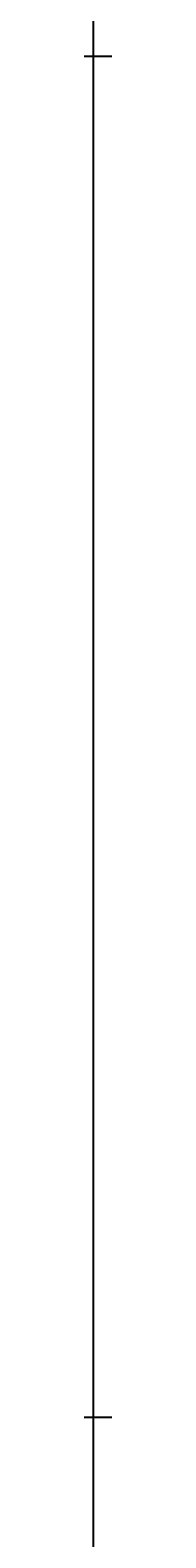
# Model space of a CAD drawing. Units: inches. Extents: x 35362 to 73946, y 43607 to 67532.
# Tile 43 of 134: x 48374 to 48377, y 46091 to 46564. Entities that reach past the tile are written whole.
import ezdxf

# ---------------------------------------------------------------- set-up
doc = ezdxf.new("R2010")
doc.units = ezdxf.units.IN
doc.header["$MEASUREMENT"] = 0
doc.layers.add('A-ANNO-DIMS', color=2, linetype='Continuous', lineweight=18)
doc.styles.get("Standard").update_dxf_attribs({"font": 'arial.ttf'})
doc.dimstyles.get("Standard").update_dxf_attribs({"dimtxt": 0.18, "dimasz": 0.18, "dimexe": 0.18, "dimexo": 0.0625, "dimgap": 0.09, "dimtad": 0, "dimtih": 1, "dimtoh": 1, "dimdec": 4, "dimzin": 0, "dimdsep": 46, "dimtxsty": 'Standard', "dimcen": 0.09, "dimadec": 0, "dimazin": 0, "dimtfac": 1, "dimtdec": 4, "dimtofl": 0, "dimtmove": 0, "dimatfit": 3, "dimfxl": 1, "dimtolj": 1, "dimtzin": 0, "dimarcsym": 0})

# ---------------------------------------------------------------- blocks, each defined once
blk = doc.blocks.new('*D5')
at = {"layer": 'A-ANNO-DIMS', "color": 0, "lineweight": -2, "transparency": 16777216}
for p, q in [((37121.95, 46919.32), (37121.95, 43606.68)), ((69871.5, 45449.83), (69871.5, 43606.68)), ((37122.13, 43606.86), (53496.29, 43606.86)), ((69871.32, 43606.86), (53497.15, 43606.86))]:
    blk.add_line(p, q, dxfattribs=at)
at = {"layer": 'A-ANNO-DIMS', "color": 0, "transparency": 16777216}
for points in [[(37122.13, 43606.89), (37122.13, 43606.83), (37121.95, 43606.86)], [(69871.32, 43606.89), (69871.32, 43606.83), (69871.5, 43606.86)]]:
    blk.add_solid(points, dxfattribs=at)
at = {"layer": 'Defpoints', "color": 0, "transparency": 16777216}
for p in [(37121.95, 46919.38), (69871.5, 45449.89), (69871.5, 43606.86)]:
    blk.add_point(p, dxfattribs=at)
at = {"layer": 'A-ANNO-DIMS', "color": 0, "transparency": 16777216, "insert": (53496.72, 43606.86), "char_height": 0.18, "attachment_point": 5}
blk.add_mtext('\\A1;32750', dxfattribs=at)
blk = doc.blocks.new('*D11')
at = {"layer": 'A-ANNO-DIMS', "color": 0, "lineweight": -2, "transparency": 16777216}
for p, q in [((47978.66, 56028.77), (47978.66, 43606.68)), ((53109.76, 56028.77), (53109.76, 43606.68)), ((47978.84, 43606.86), (50543.87, 43606.86)), ((53109.58, 43606.86), (50544.55, 43606.86))]:
    blk.add_line(p, q, dxfattribs=at)
at = {"layer": 'A-ANNO-DIMS', "color": 0, "transparency": 16777216}
for points in [[(47978.84, 43606.89), (47978.84, 43606.83), (47978.66, 43606.86)], [(53109.58, 43606.89), (53109.58, 43606.83), (53109.76, 43606.86)]]:
    blk.add_solid(points, dxfattribs=at)
at = {"layer": 'Defpoints', "color": 0, "transparency": 16777216}
for p in [(47978.66, 56028.84), (53109.76, 56028.84), (53109.76, 43606.86)]:
    blk.add_point(p, dxfattribs=at)
at = {"layer": 'A-ANNO-DIMS', "color": 0, "transparency": 16777216, "insert": (50544.21, 43606.86), "char_height": 0.18, "attachment_point": 5}
blk.add_mtext('\\A1;5131', dxfattribs=at)
blk = doc.blocks.new('*D13')
at = {"layer": 'A-ANNO-DIMS', "color": 0, "lineweight": -2, "transparency": 16777216}
for p, q in [((48373.49, 51694.02), (48373.49, 43606.68)), ((51029.04, 51694.02), (51029.04, 43606.68)), ((48373.67, 43606.86), (49700.8, 43606.86)), ((51028.86, 43606.86), (49701.73, 43606.86))]:
    blk.add_line(p, q, dxfattribs=at)
at = {"layer": 'A-ANNO-DIMS', "color": 0, "transparency": 16777216}
for points in [[(48373.67, 43606.89), (48373.67, 43606.83), (48373.49, 43606.86)], [(51028.86, 43606.89), (51028.86, 43606.83), (51029.04, 43606.86)]]:
    blk.add_solid(points, dxfattribs=at)
at = {"layer": 'Defpoints', "color": 0, "transparency": 16777216}
for p in [(48373.49, 51694.09), (51029.04, 51694.09), (51029.04, 43606.86)]:
    blk.add_point(p, dxfattribs=at)
at = {"layer": 'A-ANNO-DIMS', "color": 0, "transparency": 16777216, "insert": (49701.27, 43606.86), "char_height": 0.18, "attachment_point": 5}
blk.add_mtext('\\A1;2655.6', dxfattribs=at)
blk = doc.blocks.new('*D67')
at = {"layer": 'A-ANNO-DIMS', "color": 0, "lineweight": -2, "transparency": 16777216}
for p, q in [((56873.54, 53351.53), (35361.77, 53351.53)), ((35361.95, 53351.35), (35361.95, 49400.89)), ((35361.95, 45450.07), (35361.95, 49400.53)), ((53793.58, 45449.89), (35361.77, 45449.89))]:
    blk.add_line(p, q, dxfattribs=at)
at = {"layer": 'A-ANNO-DIMS', "color": 0, "transparency": 16777216}
for points in [[(35361.92, 53351.35), (35361.98, 53351.35), (35361.95, 53351.53)], [(35361.92, 45450.07), (35361.98, 45450.07), (35361.95, 45449.89)]]:
    blk.add_solid(points, dxfattribs=at)
at = {"layer": 'Defpoints', "color": 0, "transparency": 16777216}
for p in [(35361.95, 53351.53), (56873.6, 53351.53), (53793.64, 45449.89)]:
    blk.add_point(p, dxfattribs=at)
at = {"layer": 'A-ANNO-DIMS', "color": 0, "transparency": 16777216, "insert": (35361.95, 49400.71), "char_height": 0.18, "attachment_point": 5}
blk.add_mtext('\\A1;7901.6', dxfattribs=at)
blk = doc.blocks.new('*D76')
at = {"layer": 'A-ANNO-DIMS', "color": 0, "lineweight": -2, "transparency": 16777216}
for p, q in [((54052.84, 46555.29), (35361.77, 46555.29)), ((35361.95, 46555.11), (35361.95, 46342.27)), ((35361.95, 46129.06), (35361.95, 46341.9)), ((53793.58, 46128.88), (35361.77, 46128.88))]:
    blk.add_line(p, q, dxfattribs=at)
at = {"layer": 'A-ANNO-DIMS', "color": 0, "transparency": 16777216}
for points in [[(35361.92, 46555.11), (35361.98, 46555.11), (35361.95, 46555.29)], [(35361.92, 46129.06), (35361.98, 46129.06), (35361.95, 46128.88)]]:
    blk.add_solid(points, dxfattribs=at)
at = {"layer": 'Defpoints', "color": 0, "transparency": 16777216}
for p in [(35361.95, 46555.29), (54052.9, 46555.29), (53793.64, 46128.88)]:
    blk.add_point(p, dxfattribs=at)
at = {"layer": 'A-ANNO-DIMS', "color": 0, "transparency": 16777216, "insert": (35361.95, 46342.09), "char_height": 0.18, "attachment_point": 5}
blk.add_mtext('\\A1;426.4', dxfattribs=at)
blk = doc.blocks.new('*D90')
at = {"layer": 'A-ANNO-DIMS', "color": 0, "lineweight": -2, "transparency": 16777216}
for p, q in [((53707.72, 47291.29), (35361.77, 47291.29)), ((35361.95, 47291.11), (35361.95, 46710.26)), ((35361.95, 46129.06), (35361.95, 46709.9)), ((53793.58, 46128.88), (35361.77, 46128.88))]:
    blk.add_line(p, q, dxfattribs=at)
at = {"layer": 'A-ANNO-DIMS', "color": 0, "transparency": 16777216}
for points in [[(35361.92, 47291.11), (35361.98, 47291.11), (35361.95, 47291.29)], [(35361.92, 46129.06), (35361.98, 46129.06), (35361.95, 46128.88)]]:
    blk.add_solid(points, dxfattribs=at)
at = {"layer": 'Defpoints', "color": 0, "transparency": 16777216}
for p in [(53707.78, 47291.29), (35361.95, 46128.88), (53793.64, 46128.88)]:
    blk.add_point(p, dxfattribs=at)
at = {"layer": 'A-ANNO-DIMS', "color": 0, "transparency": 16777216, "insert": (35361.95, 46710.08), "char_height": 0.18, "attachment_point": 5}
blk.add_mtext('\\A1;1162.4', dxfattribs=at)

msp = doc.modelspace()

# ---------------------------------------------------------------- dimensions: what is measured, and where the dimension line sits
at = {"layer": 'A-ANNO-DIMS'}
for base, p1, p2, override, picture, middle in [((53109.76, 43606.859), (47978.665, 56028.836), (53109.76, 56028.836), {"dimdec": 0, "dimlfac": 1, "dimrnd": 0, "dimzin": 0, "dimdsep": 46, "dimlunit": 2}, '*D11', (50544.212, 43606.859)), ((51029.043, 43606.859), (48373.492, 51694.087), (51029.043, 51694.087), {"dimdec": 1, "dimlfac": 1, "dimrnd": 0, "dimzin": 0, "dimdsep": 46, "dimlunit": 2}, '*D13', (49701.267, 43606.859)), ((69871.496, 43606.859), (37121.949, 46919.381), (69871.496, 45449.894), {"dimdec": 0, "dimlfac": 1, "dimrnd": 0, "dimzin": 0, "dimdsep": 46, "dimlunit": 2}, '*D5', (53496.723, 43606.859))]:
    dim = msp.add_linear_dim(base=base, p1=p1, p2=p2, dimstyle='Standard', override=override, dxfattribs=at)
    dim.commit()
    dim.dimension.update_dxf_attribs({"geometry": picture, "text_midpoint": middle})
for base, p1, p2, picture, middle in [((35361.949, 53351.529), (53793.638, 45449.894), (56873.602, 53351.529), '*D67', (35361.949, 49400.712)), ((35361.949, 46128.878), (53707.781, 47291.285), (53793.638, 46128.878), '*D90', (35361.949, 46710.081)), ((35361.949, 46555.293), (53793.638, 46128.878), (54052.899, 46555.293), '*D76', (35361.949, 46342.086))]:
    dim = msp.add_linear_dim(base=base, p1=p1, p2=p2, angle=90, dimstyle='Standard', override={"dimdec": 1, "dimlfac": 1, "dimrnd": 0, "dimzin": 0, "dimdsep": 46, "dimlunit": 2}, dxfattribs=at)
    dim.commit()
    dim.dimension.update_dxf_attribs({"geometry": picture, "text_midpoint": middle})

doc.saveas('drawing.dxf')
